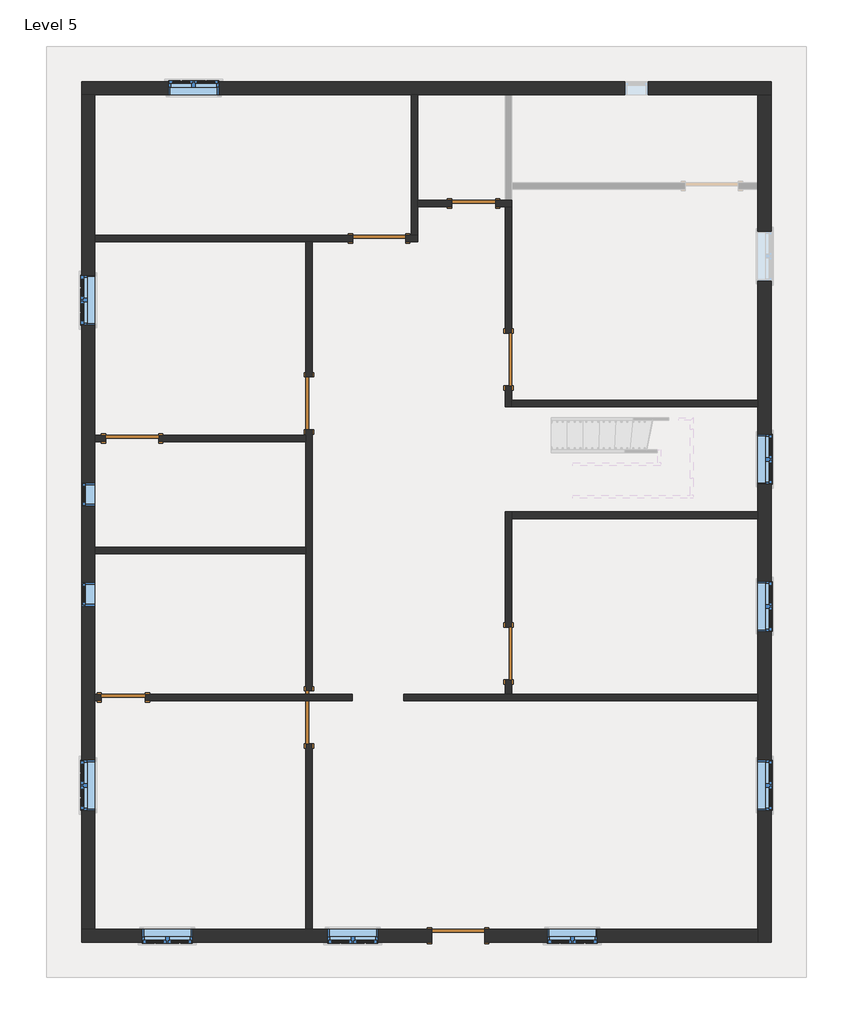
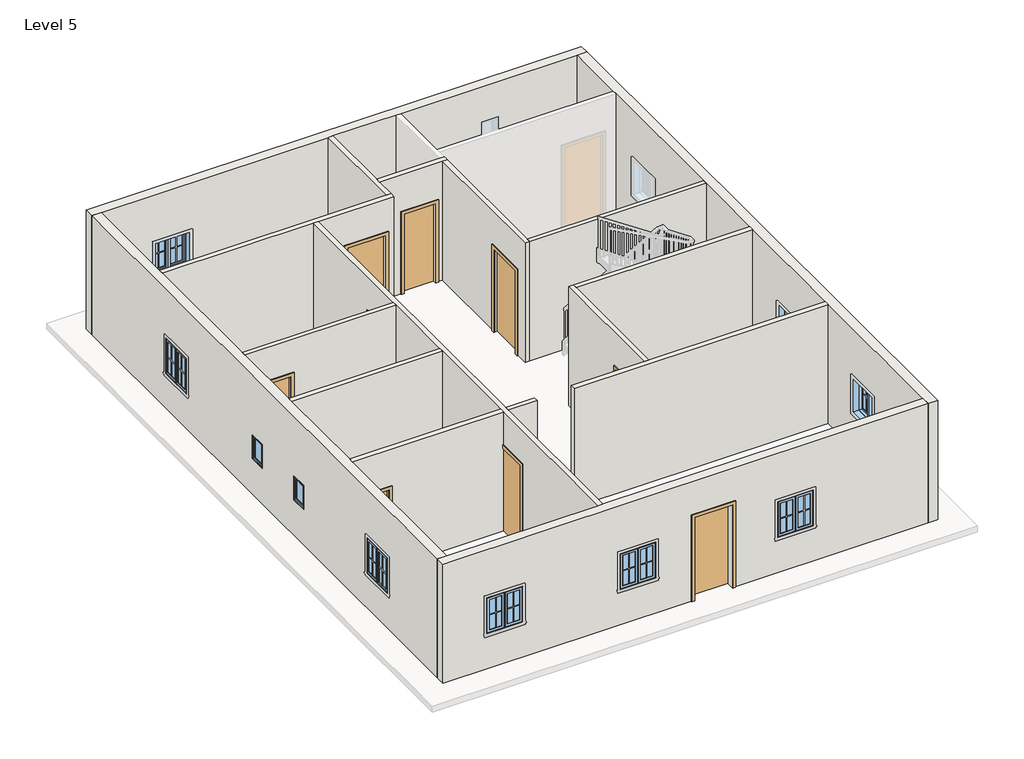
# One storey, part 1 of 3: 16 walls, 11 windows, 9 doors.
"""IFC4 building model written with IfcOpenShell, lengths in millimetres."""

from ifc_helpers import new_model, si_unit, frame, origin, place, context, project, spatial, polyline, outline, extrude, faceted_brep, transform, mapped, element, save
from components import door_d8f5dbb5, door_f2b275c1, door_e5f9f3c4, door_305aa2a5, door_a90ba1ad, window_aa618e30, window_339605e1

model = new_model("IFC4")

# Units and contexts
model_context = context("Model", 3, world=origin())
ifc_project = project(units=[si_unit("LENGTHUNIT", "METRE", prefix="MILLI")], contexts=[model_context])

# Site, building, storey
site = spatial("IfcSite", under=ifc_project)
building = spatial("IfcBuilding", under=site)
storey = spatial("IfcBuildingStorey", under=building, Name="Level 5", Elevation=9601.2)

# Doors
placement = place(None, origin())
door_shape = door_d8f5dbb5(model_context)
element("IfcDoor", 1, ObjectType="Single-Flush : 30\" x 80\"", at=placement, inside=storey, context=model_context, shape_type="MappedRepresentation", body=[
    mapped(door_shape, transform((-509.1743007, 6967.427558, 9601.2), x_axis=(1.0, 0.0, 0.0), y_axis=(0.0, 1.0, 0.0), z_axis=(0.0, 0.0, 1.0))),
])
door_2_shape = door_f2b275c1(model_context)
element("IfcDoor", 2, ObjectType="Single-Flush : 30\" x 80\"", at=placement, inside=storey, context=model_context, shape_type="MappedRepresentation", body=[
    mapped(door_2_shape, transform((-6586.1243007, -1605.072442, 9601.2), x_axis=(-1.0, 0.0, 0.0), y_axis=(0.0, -1.0, 0.0), z_axis=(0.0, 0.0, 1.0))),
])
door_3_shape = door_e5f9f3c4(model_context)
element("IfcDoor", 3, ObjectType="Single-Flush : 36\" x 84\"", at=placement, inside=storey, context=model_context, shape_type="MappedRepresentation", body=[
    mapped(door_3_shape, transform((-2147.4743007, 6357.827558, 9601.2), x_axis=(1.0, 0.0, 0.0), y_axis=(0.0, 1.0, 0.0), z_axis=(0.0, 0.0, 1.0))),
])
element("IfcDoor", 4, ObjectType="Single-Flush : 36\" x 84\"", at=placement, inside=storey, context=model_context, shape_type="MappedRepresentation", body=[
    mapped(door_3_shape, transform((100.4256993, 4262.327558, 9601.2), x_axis=(0.0, -1.0, 0.0), y_axis=(1.0, 0.0, 0.0), z_axis=(0.0, 0.0, 1.0))),
])
element("IfcDoor", 5, ObjectType="Single-Flush : 36\" x 84\"", at=placement, inside=storey, context=model_context, shape_type="MappedRepresentation", body=[
    mapped(door_3_shape, transform((100.4256993, -843.072442, 9601.2), x_axis=(0.0, -1.0, 0.0), y_axis=(1.0, 0.0, 0.0), z_axis=(0.0, 0.0, 1.0))),
])
element("IfcDoor", 6, ObjectType="Single-Flush : 36\" x 84\"", at=placement, inside=storey, context=model_context, shape_type="MappedRepresentation", body=[
    mapped(door_3_shape, transform((-3366.6743007, -1947.972442, 9601.2), x_axis=(0.0, 1.0, 0.0), y_axis=(-1.0, 0.0, 0.0), z_axis=(0.0, 0.0, 1.0))),
])
door_4_shape = door_305aa2a5(model_context)
element("IfcDoor", 7, ObjectType="Single-Flush : 36\" x 84\"", at=placement, inside=storey, context=model_context, shape_type="MappedRepresentation", body=[
    mapped(door_4_shape, transform((-6433.7243007, 2890.727558, 9601.2), x_axis=(-1.0, 0.0, 0.0), y_axis=(0.0, -1.0, 0.0), z_axis=(0.0, 0.0, 1.0))),
])
element("IfcDoor", 8, ObjectType="Single-Flush : 36\" x 84\"", at=placement, inside=storey, context=model_context, shape_type="MappedRepresentation", body=[
    mapped(door_4_shape, transform((-3366.6743007, 3500.327558, 9601.2), x_axis=(0.0, -1.0, 0.0), y_axis=(1.0, 0.0, 0.0), z_axis=(0.0, 0.0, 1.0))),
])
door_5_shape = door_a90ba1ad(model_context)
element("IfcDoor", 9, ObjectType="Single-Flush : 36\" x 84\"", at=placement, inside=storey, context=model_context, shape_type="MappedRepresentation", body=[
    mapped(door_5_shape, transform((-775.8743007, -5738.922442, 9601.2), x_axis=(-1.0, 0.0, 0.0), y_axis=(0.0, -1.0, 0.0), z_axis=(0.0, 0.0, 1.0))),
])

# Walls
element("IfcWall", 10, ObjectType="WALL4.5\"", at=placement, inside=storey, context=model_context, shape_type="Brep", body=[
    faceted_brep([(-1690.2743007, 6300.677558, 11734.8), (-1690.2743007, 6300.677558, 9601.2), (-1480.7243007, 6300.677558, 9601.2), (-1480.7243007, 6300.677558, 12649.2), (-3309.5243007, 6300.677558, 12649.2), (-3423.8243007, 6300.677558, 12649.2), (-7081.4243007, 6300.677558, 12649.2), (-7081.4243007, 6300.677558, 9601.2), (-3423.8243007, 6300.677558, 9601.2), (-3309.5243007, 6300.677558, 9601.2), (-2604.6743007, 6300.677558, 9601.2), (-2604.6743007, 6300.677558, 11734.8), (-1480.7243007, 6414.977558, 9601.2), (-1595.0243007, 6414.977558, 9601.2), (-1690.2743007, 6414.977558, 9601.2), (-1690.2743007, 6414.977558, 11734.8), (-2604.6743007, 6414.977558, 11734.8), (-2604.6743007, 6414.977558, 9601.2), (-7081.4243007, 6414.977558, 9601.2), (-7081.4243007, 6414.977558, 12649.2), (-1595.0243007, 6414.977558, 12649.2), (-1480.7243007, 6414.977558, 12649.2)], [[[0, 1, 2, 3, 4, 5, 6, 7, 8, 9, 10, 11]], [[12, 13, 14, 15, 16, 17, 18, 19, 20, 21]], [[2, 1, 14, 13, 12]], [[10, 9, 8, 7, 18, 17]], [[7, 6, 19, 18]], [[3, 2, 12, 21]], [[15, 14, 1, 0]], [[16, 15, 0, 11]], [[17, 16, 11, 10]], [[6, 5, 4, 3, 21, 20, 19]]]),
])
element("IfcWall", 11, ObjectType="WALL4.5\"", at=placement, inside=storey, context=model_context, shape_type="Brep", body=[
    faceted_brep([(-1480.7243007, 6414.977558, 9601.2), (-1480.7243007, 6910.277558, 9601.2), (-1480.7243007, 7024.577558, 9601.2), (-1480.7243007, 8853.377558, 9601.2), (-1480.7243007, 8853.377558, 12649.2), (-1480.7243007, 7024.577558, 12649.2), (-1480.7243007, 6910.277558, 12649.2), (-1480.7243007, 6414.977558, 12649.2), (-1595.0243007, 6414.977558, 9601.2), (-1595.0243007, 6414.977558, 12649.2), (-1595.0243007, 8853.377558, 12649.2), (-1595.0243007, 8853.377558, 9601.2)], [[[0, 1, 2, 3, 4, 5, 6, 7]], [[8, 9, 10, 11]], [[3, 2, 1, 0, 8, 11]], [[0, 7, 9, 8]], [[4, 3, 11, 10]], [[7, 6, 5, 4, 10, 9]]]),
])
element("IfcWall", 12, ObjectType="WALL4.5\"", at=placement, inside=storey, context=model_context, shape_type="Brep", body=[
    faceted_brep([(-128.1743007, 6910.277558, 11633.2), (-128.1743007, 6910.277558, 9601.2), (43.2756993, 6910.277558, 9601.2), (157.5756993, 6910.277558, 9601.2), (157.5756993, 6910.277558, 12649.2), (43.2756993, 6910.277558, 12649.2), (-1480.7243007, 6910.277558, 12649.2), (-1480.7243007, 6910.277558, 9601.2), (-890.1743007, 6910.277558, 9601.2), (-890.1743007, 6910.277558, 11633.2), (157.5756993, 7024.577558, 9601.2), (43.2756993, 7024.577558, 9601.2), (-128.1743007, 7024.577558, 9601.2), (-128.1743007, 7024.577558, 11633.2), (-890.1743007, 7024.577558, 11633.2), (-890.1743007, 7024.577558, 9601.2), (-1480.7243007, 7024.577558, 9601.2), (-1480.7243007, 7024.577558, 12649.2), (43.2756993, 7024.577558, 12649.2), (157.5756993, 7024.577558, 12649.2)], [[[0, 1, 2, 3, 4, 5, 6, 7, 8, 9]], [[10, 11, 12, 13, 14, 15, 16, 17, 18, 19]], [[8, 7, 16, 15]], [[3, 2, 1, 12, 11, 10]], [[7, 6, 17, 16]], [[4, 3, 10, 19]], [[13, 12, 1, 0]], [[14, 13, 0, 9]], [[15, 14, 9, 8]], [[6, 5, 4, 19, 18, 17]]]),
])
element("IfcWall", 13, ObjectType="WALL4.5\"", at=placement, inside=storey, context=model_context, shape_type="Brep", body=[
    faceted_brep([(-3423.8243007, 3043.127558, 9601.2), (-3423.8243007, 2947.877558, 9601.2), (-3423.8243007, 2833.577558, 9601.2), (-3423.8243007, 1004.777558, 9601.2), (-3423.8243007, 890.477558, 9601.2), (-3423.8243007, -1490.772442, 9601.2), (-3423.8243007, -1490.772442, 11734.8), (-3423.8243007, -1547.922442, 11734.8), (-3423.8243007, -1662.222442, 11734.8), (-3423.8243007, -2405.172442, 11734.8), (-3423.8243007, -2405.172442, 9601.2), (-3423.8243007, -5624.622442, 9601.2), (-3423.8243007, -5624.622442, 12649.2), (-3423.8243007, -1662.222442, 12649.2), (-3423.8243007, -1547.922442, 12649.2), (-3423.8243007, 890.477558, 12649.2), (-3423.8243007, 1004.777558, 12649.2), (-3423.8243007, 2833.577558, 12649.2), (-3423.8243007, 2947.877558, 12649.2), (-3423.8243007, 6300.677558, 12649.2), (-3423.8243007, 6300.677558, 9601.2), (-3423.8243007, 3957.527558, 9601.2), (-3423.8243007, 3957.527558, 11734.8), (-3423.8243007, 3043.127558, 11734.8), (-3309.5243007, -1490.772442, 11734.8), (-3309.5243007, -1490.772442, 9601.2), (-3309.5243007, 3043.127558, 9601.2), (-3309.5243007, 3043.127558, 11734.8), (-3309.5243007, 3957.527558, 11734.8), (-3309.5243007, 3957.527558, 9601.2), (-3309.5243007, 6300.677558, 9601.2), (-3309.5243007, 6300.677558, 12649.2), (-3309.5243007, -1547.922442, 12649.2), (-3309.5243007, -1662.222442, 12649.2), (-3309.5243007, -5624.622442, 12649.2), (-3309.5243007, -5624.622442, 9601.2), (-3309.5243007, -2405.172442, 9601.2), (-3309.5243007, -2405.172442, 11734.8), (-3309.5243007, -1662.222442, 11734.8), (-3309.5243007, -1547.922442, 11734.8)], [[[0, 1, 2, 3, 4, 5, 6, 7, 8, 9, 10, 11, 12, 13, 14, 15, 16, 17, 18, 19, 20, 21, 22, 23]], [[24, 25, 26, 27, 28, 29, 30, 31, 32, 33, 34, 35, 36, 37, 38, 39]], [[21, 20, 30, 29]], [[36, 35, 11, 10]], [[26, 25, 5, 4, 3, 2, 1, 0]], [[12, 11, 35, 34]], [[20, 19, 31, 30]], [[27, 26, 0, 23]], [[28, 27, 23, 22]], [[29, 28, 22, 21]], [[6, 5, 25, 24]], [[9, 8, 7, 6, 24, 39, 38, 37]], [[10, 9, 37, 36]], [[19, 18, 17, 16, 15, 14, 13, 12, 34, 33, 32, 31]]]),
])
element("IfcWall", 14, ObjectType="WALL4.5\"", at=placement, inside=storey, context=model_context, shape_type="Brep", body=[
    faceted_brep([(157.5756993, -1547.922442, 9601.2), (157.5756993, -1300.272442, 9601.2), (157.5756993, -1300.272442, 11734.8), (157.5756993, -385.872442, 11734.8), (157.5756993, -385.872442, 9601.2), (157.5756993, 1500.077558, 9601.2), (157.5756993, 1614.377558, 9601.2), (157.5756993, 1614.377558, 12649.2), (157.5756993, 1500.077558, 12649.2), (157.5756993, -1547.922442, 12649.2), (43.2756993, -1300.272442, 11734.8), (43.2756993, -1300.272442, 9601.2), (43.2756993, -1547.922442, 9601.2), (43.2756993, -1547.922442, 12649.2), (43.2756993, 1614.377558, 12649.2), (43.2756993, 1614.377558, 9601.2), (43.2756993, -385.872442, 9601.2), (43.2756993, -385.872442, 11734.8)], [[[0, 1, 2, 3, 4, 5, 6, 7, 8, 9]], [[10, 11, 12, 13, 14, 15, 16, 17]], [[16, 15, 6, 5, 4]], [[12, 11, 1, 0]], [[7, 6, 15, 14]], [[0, 9, 13, 12]], [[2, 1, 11, 10]], [[3, 2, 10, 17]], [[4, 3, 17, 16]], [[9, 8, 7, 14, 13]]]),
])
element("IfcWall", 15, ObjectType="WALL4.5\"", at=placement, inside=storey, context=model_context, shape_type="SweptSolid", body=[
    extrude(outline(polyline([(4424.7756993, 1500.077558), (157.5756993, 1500.077558), (157.5756993, 1614.377558), (4424.7756993, 1614.377558), (4424.7756993, 1500.077558)])), frame((0.0, 0.0, 9601.2), z_axis=(0.0, 0.0, 1.0), x_axis=(1.0, 0.0, 0.0)), (0.0, 0.0, 1.0), 3048.0),
])
element("IfcWall", 16, ObjectType="WALL4.5\"", at=placement, inside=storey, context=model_context, shape_type="SweptSolid", body=[
    extrude(outline(polyline([(-3423.8243007, 890.477558), (-7081.4243007, 890.477558), (-7081.4243007, 1004.777558), (-3423.8243007, 1004.777558), (-3423.8243007, 890.477558)])), frame((0.0, 0.0, 9601.2), z_axis=(0.0, 0.0, 1.0), x_axis=(1.0, 0.0, 0.0)), (0.0, 0.0, 1.0), 3048.0),
])
element("IfcWall", 17, ObjectType="WALL4.5\"", at=placement, inside=storey, context=model_context, shape_type="SweptSolid", body=[
    extrude(outline(polyline([(9601.2, -7081.4243007), (9601.2, -6890.9243007), (11734.8, -6890.9243007), (11734.8, -5976.5243007), (9601.2, -5976.5243007), (9601.2, -3423.8243007), (12649.2, -3423.8243007), (12649.2, -7081.4243007), (9601.2, -7081.4243007)])), frame((0.0, 2833.577558, 0.0), z_axis=(0.0, 1.0, 0.0), x_axis=(0.0, 0.0, 1.0)), (0.0, 0.0, 1.0), 114.3),
])
element("IfcWall", 18, ObjectType="WALL4.5\"", at=placement, inside=storey, context=model_context, shape_type="Brep", body=[
    faceted_brep([(43.2756993, 3805.127558, 11734.8), (43.2756993, 3805.127558, 9601.2), (43.2756993, 3443.177558, 9601.2), (43.2756993, 3443.177558, 12649.2), (43.2756993, 6910.277558, 12649.2), (43.2756993, 6910.277558, 9601.2), (43.2756993, 4719.527558, 9601.2), (43.2756993, 4719.527558, 11734.8), (157.5756993, 3443.177558, 9601.2), (157.5756993, 3557.477558, 9601.2), (157.5756993, 3805.127558, 9601.2), (157.5756993, 3805.127558, 11734.8), (157.5756993, 4719.527558, 11734.8), (157.5756993, 4719.527558, 9601.2), (157.5756993, 6910.277558, 9601.2), (157.5756993, 6910.277558, 12649.2), (157.5756993, 3557.477558, 12649.2), (157.5756993, 3443.177558, 12649.2)], [[[0, 1, 2, 3, 4, 5, 6, 7]], [[8, 9, 10, 11, 12, 13, 14, 15, 16, 17]], [[6, 5, 14, 13]], [[2, 1, 10, 9, 8]], [[5, 4, 15, 14]], [[3, 2, 8, 17]], [[11, 10, 1, 0]], [[12, 11, 0, 7]], [[13, 12, 7, 6]], [[4, 3, 17, 16, 15]]]),
])
element("IfcWall", 19, ObjectType="WALL4.5\"", at=placement, inside=storey, context=model_context, shape_type="SweptSolid", body=[
    extrude(outline(polyline([(4424.7756993, 3443.177558), (157.5756993, 3443.177558), (157.5756993, 3557.477558), (4424.7756993, 3557.477558), (4424.7756993, 3443.177558)])), frame((0.0, 0.0, 9601.2), z_axis=(0.0, 0.0, 1.0), x_axis=(1.0, 0.0, 0.0)), (0.0, 0.0, 1.0), 3048.0),
])
element("IfcWall", 20, ObjectType="WALL4.5\"", at=placement, inside=storey, context=model_context, shape_type="SweptSolid", body=[
    extrude(outline(polyline([(9601.2, -2614.8628774), (12649.2, -2614.8628774), (12649.2, -3309.5243007), (11734.8, -3309.5243007), (11734.8, -3423.8243007), (12649.2, -3423.8243007), (12649.2, -7081.4243007), (9601.2, -7081.4243007), (9601.2, -6967.1243007), (11633.2, -6967.1243007), (11633.2, -6205.1243007), (9601.2, -6205.1243007), (9601.2, -2614.8628774)])), frame((0.0, -1662.222442, 0.0), z_axis=(0.0, 1.0, 0.0), x_axis=(0.0, 0.0, 1.0)), (0.0, 0.0, 1.0), 114.3),
])
element("IfcWall", 21, ObjectType="WALL4.5\"", at=placement, inside=storey, context=model_context, shape_type="Brep", body=[
    faceted_brep([(-1720.6441625, -1662.222442, 9601.2), (4424.7756993, -1662.222442, 9601.2), (4424.7756993, -1662.222442, 12649.2), (-1720.6441625, -1662.222442, 12649.2), (-1720.6441625, -1547.922442, 9601.2), (-1720.6441625, -1547.922442, 12649.2), (43.2756993, -1547.922442, 12649.2), (157.5756993, -1547.922442, 12649.2), (4424.7756993, -1547.922442, 12649.2), (4424.7756993, -1547.922442, 9601.2), (157.5756993, -1547.922442, 9601.2), (43.2756993, -1547.922442, 9601.2)], [[[0, 1, 2, 3]], [[4, 5, 6, 7, 8, 9, 10, 11]], [[1, 0, 4, 11, 10, 9]], [[0, 3, 5, 4]], [[2, 1, 9, 8]], [[3, 2, 8, 7, 6, 5]]]),
])
element("IfcWall", 22, ObjectType="WALL9\"", at=placement, inside=storey, context=model_context, shape_type="Brep", body=[
    faceted_brep([(-7310.0243007, 8853.377558, 9601.2), (-7081.4243007, 8853.377558, 9601.2), (-1595.0243007, 8853.377558, 9601.2), (-1480.7243007, 8853.377558, 9601.2), (43.2756993, 8853.377558, 9601.2), (157.5756993, 8853.377558, 9601.2), (4424.7756993, 8853.377558, 9601.2), (4653.3756993, 8853.377558, 9601.2), (4653.3756993, 8853.377558, 12649.2), (4424.7756993, 8853.377558, 12649.2), (157.5756993, 8853.377558, 12649.2), (43.2756993, 8853.377558, 12649.2), (-1480.7243007, 8853.377558, 12649.2), (-1595.0243007, 8853.377558, 12649.2), (-7081.4243007, 8853.377558, 12649.2), (-7310.0243007, 8853.377558, 12649.2), (-4935.1243007, 8853.377558, 11430.0), (-4935.1243007, 8853.377558, 10515.6), (-5798.7243007, 8853.377558, 10515.6), (-5798.7243007, 8853.377558, 11430.0), (2522.9506993, 8853.377558, 11734.8), (2522.9506993, 8853.377558, 9906.0), (2116.5506993, 8853.377558, 9906.0), (2116.5506993, 8853.377558, 11734.8), (-7310.0243007, 9081.977558, 9601.2), (-7310.0243007, 9081.977558, 12649.2), (4653.3756993, 9081.977558, 12649.2), (4653.3756993, 9081.977558, 9601.2), (-4935.1243007, 9081.977558, 11430.0), (-5798.7243007, 9081.977558, 11430.0), (-5798.7243007, 9081.977558, 10515.6), (-4935.1243007, 9081.977558, 10515.6), (2522.9506993, 9081.977558, 11734.8), (2116.5506993, 9081.977558, 11734.8), (2116.5506993, 9081.977558, 9906.0), (2522.9506993, 9081.977558, 9906.0)], [[[0, 1, 2, 3, 4, 5, 6, 7, 8, 9, 10, 11, 12, 13, 14, 15], [16, 17, 18, 19], [20, 21, 22, 23]], [[24, 25, 26, 27], [28, 29, 30, 31], [32, 33, 34, 35]], [[7, 6, 5, 4, 3, 2, 1, 0, 24, 27]], [[8, 7, 27, 26]], [[0, 15, 25, 24]], [[17, 16, 28, 31]], [[18, 17, 31, 30]], [[19, 18, 30, 29]], [[16, 19, 29, 28]], [[21, 20, 32, 35]], [[22, 21, 35, 34]], [[23, 22, 34, 33]], [[20, 23, 33, 32]], [[15, 14, 13, 12, 11, 10, 9, 8, 26, 25]]]),
])
element("IfcWall", 23, ObjectType="WALL9\"", at=placement, inside=storey, context=model_context, shape_type="Brep", body=[
    faceted_brep([(4424.7756993, 8853.377558, 9601.2), (4424.7756993, 7329.377558, 9601.2), (4424.7756993, 7215.077558, 9601.2), (4424.7756993, 3557.477558, 9601.2), (4424.7756993, 3443.177558, 9601.2), (4424.7756993, 1614.377558, 9601.2), (4424.7756993, 1500.077558, 9601.2), (4424.7756993, -1547.922442, 9601.2), (4424.7756993, -1662.222442, 9601.2), (4424.7756993, -5624.622442, 9601.2), (4424.7756993, -5853.222442, 9601.2), (4424.7756993, -5853.222442, 12649.2), (4424.7756993, -5624.622442, 12649.2), (4424.7756993, -1662.222442, 12649.2), (4424.7756993, -1547.922442, 12649.2), (4424.7756993, 1500.077558, 12649.2), (4424.7756993, 1614.377558, 12649.2), (4424.7756993, 3443.177558, 12649.2), (4424.7756993, 3557.477558, 12649.2), (4424.7756993, 7215.077558, 12649.2), (4424.7756993, 7329.377558, 12649.2), (4424.7756993, 8853.377558, 12649.2), (4424.7756993, 5621.227558, 11430.0), (4424.7756993, 5621.227558, 10515.6), (4424.7756993, 6484.827558, 10515.6), (4424.7756993, 6484.827558, 11430.0), (4424.7756993, 2096.977558, 11430.0), (4424.7756993, 2096.977558, 10515.6), (4424.7756993, 2960.577558, 10515.6), (4424.7756993, 2960.577558, 11430.0), (4424.7756993, -455.722442, 11430.0), (4424.7756993, -455.722442, 10515.6), (4424.7756993, 407.877558, 10515.6), (4424.7756993, 407.877558, 11430.0), (4424.7756993, -3560.872442, 11430.0), (4424.7756993, -3560.872442, 10515.6), (4424.7756993, -2697.272442, 10515.6), (4424.7756993, -2697.272442, 11430.0), (4653.3756993, 8853.377558, 9601.2), (4653.3756993, 8853.377558, 12649.2), (4653.3756993, -5853.222442, 12649.2), (4653.3756993, -5853.222442, 9601.2), (4653.3756993, 5621.227558, 11430.0), (4653.3756993, 6484.827558, 11430.0), (4653.3756993, 6484.827558, 10515.6), (4653.3756993, 5621.227558, 10515.6), (4653.3756993, 2096.977558, 11430.0), (4653.3756993, 2960.577558, 11430.0), (4653.3756993, 2960.577558, 10515.6), (4653.3756993, 2096.977558, 10515.6), (4653.3756993, -455.722442, 11430.0), (4653.3756993, 407.877558, 11430.0), (4653.3756993, 407.877558, 10515.6), (4653.3756993, -455.722442, 10515.6), (4653.3756993, -3560.872442, 11430.0), (4653.3756993, -2697.272442, 11430.0), (4653.3756993, -2697.272442, 10515.6), (4653.3756993, -3560.872442, 10515.6)], [[[0, 1, 2, 3, 4, 5, 6, 7, 8, 9, 10, 11, 12, 13, 14, 15, 16, 17, 18, 19, 20, 21], [22, 23, 24, 25], [26, 27, 28, 29], [30, 31, 32, 33], [34, 35, 36, 37]], [[38, 39, 40, 41], [42, 43, 44, 45], [46, 47, 48, 49], [50, 51, 52, 53], [54, 55, 56, 57]], [[10, 9, 8, 7, 6, 5, 4, 3, 2, 1, 0, 38, 41]], [[0, 21, 39, 38]], [[11, 10, 41, 40]], [[23, 22, 42, 45]], [[24, 23, 45, 44]], [[25, 24, 44, 43]], [[22, 25, 43, 42]], [[27, 26, 46, 49]], [[28, 27, 49, 48]], [[29, 28, 48, 47]], [[26, 29, 47, 46]], [[31, 30, 50, 53]], [[32, 31, 53, 52]], [[33, 32, 52, 51]], [[30, 33, 51, 50]], [[35, 34, 54, 57]], [[36, 35, 57, 56]], [[37, 36, 56, 55]], [[34, 37, 55, 54]], [[21, 20, 19, 18, 17, 16, 15, 14, 13, 12, 11, 40, 39]]]),
])
element("IfcWall", 24, ObjectType="WALL9\"", at=placement, inside=storey, context=model_context, shape_type="Brep", body=[
    faceted_brep([(-1233.0743007, -5624.622442, 11734.8), (-1233.0743007, -5624.622442, 9601.2), (-3309.5243007, -5624.622442, 9601.2), (-3423.8243007, -5624.622442, 9601.2), (-7081.4243007, -5624.622442, 9601.2), (-7310.0243007, -5624.622442, 9601.2), (-7310.0243007, -5624.622442, 12649.2), (-7081.4243007, -5624.622442, 12649.2), (-3423.8243007, -5624.622442, 12649.2), (-3309.5243007, -5624.622442, 12649.2), (4424.7756993, -5624.622442, 12649.2), (4424.7756993, -5624.622442, 9601.2), (-318.6743007, -5624.622442, 9601.2), (-318.6743007, -5624.622442, 11734.8), (773.5256993, -5624.622442, 11430.0), (773.5256993, -5624.622442, 10515.6), (1637.1256993, -5624.622442, 10515.6), (1637.1256993, -5624.622442, 11430.0), (-3036.4743007, -5624.622442, 11430.0), (-3036.4743007, -5624.622442, 10515.6), (-2172.8743007, -5624.622442, 10515.6), (-2172.8743007, -5624.622442, 11430.0), (-6255.9243007, -5624.622442, 11430.0), (-6255.9243007, -5624.622442, 10515.6), (-5392.3243007, -5624.622442, 10515.6), (-5392.3243007, -5624.622442, 11430.0), (-7310.0243007, -5853.222442, 9601.2), (-1233.0743007, -5853.222442, 9601.2), (-1233.0743007, -5853.222442, 11734.8), (-318.6743007, -5853.222442, 11734.8), (-318.6743007, -5853.222442, 9601.2), (4424.7756993, -5853.222442, 9601.2), (4424.7756993, -5853.222442, 12649.2), (-7310.0243007, -5853.222442, 12649.2), (773.5256993, -5853.222442, 11430.0), (1637.1256993, -5853.222442, 11430.0), (1637.1256993, -5853.222442, 10515.6), (773.5256993, -5853.222442, 10515.6), (-3036.4743007, -5853.222442, 11430.0), (-2172.8743007, -5853.222442, 11430.0), (-2172.8743007, -5853.222442, 10515.6), (-3036.4743007, -5853.222442, 10515.6), (-6255.9243007, -5853.222442, 11430.0), (-5392.3243007, -5853.222442, 11430.0), (-5392.3243007, -5853.222442, 10515.6), (-6255.9243007, -5853.222442, 10515.6)], [[[0, 1, 2, 3, 4, 5, 6, 7, 8, 9, 10, 11, 12, 13], [14, 15, 16, 17], [18, 19, 20, 21], [22, 23, 24, 25]], [[26, 27, 28, 29, 30, 31, 32, 33], [34, 35, 36, 37], [38, 39, 40, 41], [42, 43, 44, 45]], [[12, 11, 31, 30]], [[5, 4, 3, 2, 1, 27, 26]], [[11, 10, 32, 31]], [[6, 5, 26, 33]], [[28, 27, 1, 0]], [[29, 28, 0, 13]], [[30, 29, 13, 12]], [[15, 14, 34, 37]], [[16, 15, 37, 36]], [[17, 16, 36, 35]], [[14, 17, 35, 34]], [[19, 18, 38, 41]], [[20, 19, 41, 40]], [[21, 20, 40, 39]], [[18, 21, 39, 38]], [[23, 22, 42, 45]], [[24, 23, 45, 44]], [[25, 24, 44, 43]], [[22, 25, 43, 42]], [[10, 9, 8, 7, 6, 33, 32]]]),
])
element("IfcWall", 25, ObjectType="WALL9\"", at=placement, inside=storey, context=model_context, shape_type="Brep", body=[
    faceted_brep([(-7081.4243007, -5624.622442, 9601.2), (-7081.4243007, -1662.222442, 9601.2), (-7081.4243007, -1547.922442, 9601.2), (-7081.4243007, 890.477558, 9601.2), (-7081.4243007, 1004.777558, 9601.2), (-7081.4243007, 2833.577558, 9601.2), (-7081.4243007, 2947.877558, 9601.2), (-7081.4243007, 6300.677558, 9601.2), (-7081.4243007, 6414.977558, 9601.2), (-7081.4243007, 8853.377558, 9601.2), (-7081.4243007, 8853.377558, 12649.2), (-7081.4243007, 6414.977558, 12649.2), (-7081.4243007, 6300.677558, 12649.2), (-7081.4243007, 2947.877558, 12649.2), (-7081.4243007, 2833.577558, 12649.2), (-7081.4243007, 1004.777558, 12649.2), (-7081.4243007, 890.477558, 12649.2), (-7081.4243007, -1547.922442, 12649.2), (-7081.4243007, -1662.222442, 12649.2), (-7081.4243007, -5624.622442, 12649.2), (-7081.4243007, 388.827558, 11125.2), (-7081.4243007, 388.827558, 10515.6), (-7081.4243007, -17.572442, 10515.6), (-7081.4243007, -17.572442, 11125.2), (-7081.4243007, 2122.377558, 11125.2), (-7081.4243007, 2122.377558, 10515.6), (-7081.4243007, 1715.977558, 10515.6), (-7081.4243007, 1715.977558, 11125.2), (-7081.4243007, 5722.827558, 11430.0), (-7081.4243007, 5722.827558, 10515.6), (-7081.4243007, 4859.227558, 10515.6), (-7081.4243007, 4859.227558, 11430.0), (-7081.4243007, -2697.272442, 11430.0), (-7081.4243007, -2697.272442, 10515.6), (-7081.4243007, -3560.872442, 10515.6), (-7081.4243007, -3560.872442, 11430.0), (-7310.0243007, -5624.622442, 9601.2), (-7310.0243007, -5624.622442, 12649.2), (-7310.0243007, 8853.377558, 12649.2), (-7310.0243007, 8853.377558, 9601.2), (-7310.0243007, 388.827558, 11125.2), (-7310.0243007, -17.572442, 11125.2), (-7310.0243007, -17.572442, 10515.6), (-7310.0243007, 388.827558, 10515.6), (-7310.0243007, 2122.377558, 11125.2), (-7310.0243007, 1715.977558, 11125.2), (-7310.0243007, 1715.977558, 10515.6), (-7310.0243007, 2122.377558, 10515.6), (-7310.0243007, 5722.827558, 11430.0), (-7310.0243007, 4859.227558, 11430.0), (-7310.0243007, 4859.227558, 10515.6), (-7310.0243007, 5722.827558, 10515.6), (-7310.0243007, -2697.272442, 11430.0), (-7310.0243007, -3560.872442, 11430.0), (-7310.0243007, -3560.872442, 10515.6), (-7310.0243007, -2697.272442, 10515.6)], [[[0, 1, 2, 3, 4, 5, 6, 7, 8, 9, 10, 11, 12, 13, 14, 15, 16, 17, 18, 19], [20, 21, 22, 23], [24, 25, 26, 27], [28, 29, 30, 31], [32, 33, 34, 35]], [[36, 37, 38, 39], [40, 41, 42, 43], [44, 45, 46, 47], [48, 49, 50, 51], [52, 53, 54, 55]], [[9, 8, 7, 6, 5, 4, 3, 2, 1, 0, 36, 39]], [[10, 9, 39, 38]], [[0, 19, 37, 36]], [[21, 20, 40, 43]], [[22, 21, 43, 42]], [[23, 22, 42, 41]], [[20, 23, 41, 40]], [[25, 24, 44, 47]], [[26, 25, 47, 46]], [[27, 26, 46, 45]], [[24, 27, 45, 44]], [[29, 28, 48, 51]], [[30, 29, 51, 50]], [[31, 30, 50, 49]], [[28, 31, 49, 48]], [[33, 32, 52, 55]], [[34, 33, 55, 54]], [[35, 34, 54, 53]], [[32, 35, 53, 52]], [[19, 18, 17, 16, 15, 14, 13, 12, 11, 10, 38, 37]]]),
])

# Windows
window_shape = window_aa618e30(model_context)
element("IfcWindow", 26, ObjectType="Fixed : 16\" x 24\"", at=placement, inside=storey, context=model_context, shape_type="MappedRepresentation", body=[
    mapped(window_shape, transform((-7195.7243007, 223.727558, 9601.2), x_axis=(0.0, 1.0, 0.0), y_axis=(-1.0, 0.0, 0.0), z_axis=(0.0, 0.0, 1.0))),
])
element("IfcWindow", 27, ObjectType="Fixed : 16\" x 24\"", at=placement, inside=storey, context=model_context, shape_type="MappedRepresentation", body=[
    mapped(window_shape, transform((-7195.7243007, 1957.277558, 9601.2), x_axis=(0.0, 1.0, 0.0), y_axis=(-1.0, 0.0, 0.0), z_axis=(0.0, 0.0, 1.0))),
])
window_2_shape = window_339605e1(model_context)
element("IfcWindow", 28, ObjectType="Window-Casement-Double : 34\" x 36\"", at=placement, inside=storey, context=model_context, shape_type="MappedRepresentation", body=[
    mapped(window_2_shape, transform((-5366.9243007, 8967.677558, 9601.2), x_axis=(1.0, 0.0, 0.0), y_axis=(0.0, 1.0, 0.0), z_axis=(0.0, 0.0, 1.0))),
])
element("IfcWindow", 29, ObjectType="Window-Casement-Double : 34\" x 36\"", at=placement, inside=storey, context=model_context, shape_type="MappedRepresentation", body=[
    mapped(window_2_shape, transform((-7195.7243007, 5291.027558, 9601.2), x_axis=(0.0, 1.0, 0.0), y_axis=(-1.0, 0.0, 0.0), z_axis=(0.0, 0.0, 1.0))),
])
element("IfcWindow", 30, ObjectType="Window-Casement-Double : 34\" x 36\"", at=placement, inside=storey, context=model_context, shape_type="MappedRepresentation", body=[
    mapped(window_2_shape, transform((4539.0756993, 2528.777558, 9601.2), x_axis=(0.0, -1.0, 0.0), y_axis=(1.0, 0.0, 0.0), z_axis=(0.0, 0.0, 1.0))),
])
element("IfcWindow", 31, ObjectType="Window-Casement-Double : 34\" x 36\"", at=placement, inside=storey, context=model_context, shape_type="MappedRepresentation", body=[
    mapped(window_2_shape, transform((4539.0756993, -23.922442, 9601.2), x_axis=(0.0, -1.0, 0.0), y_axis=(1.0, 0.0, 0.0), z_axis=(0.0, 0.0, 1.0))),
])
element("IfcWindow", 32, ObjectType="Window-Casement-Double : 34\" x 36\"", at=placement, inside=storey, context=model_context, shape_type="MappedRepresentation", body=[
    mapped(window_2_shape, transform((4539.0756993, -3129.072442, 9601.2), x_axis=(0.0, -1.0, 0.0), y_axis=(1.0, 0.0, 0.0), z_axis=(0.0, 0.0, 1.0))),
])
element("IfcWindow", 33, ObjectType="Window-Casement-Double : 34\" x 36\"", at=placement, inside=storey, context=model_context, shape_type="MappedRepresentation", body=[
    mapped(window_2_shape, transform((1205.3256993, -5738.922442, 9601.2), x_axis=(-1.0, 0.0, 0.0), y_axis=(0.0, -1.0, 0.0), z_axis=(0.0, 0.0, 1.0))),
])
element("IfcWindow", 34, ObjectType="Window-Casement-Double : 34\" x 36\"", at=placement, inside=storey, context=model_context, shape_type="MappedRepresentation", body=[
    mapped(window_2_shape, transform((-2604.6743007, -5738.922442, 9601.2), x_axis=(-1.0, 0.0, 0.0), y_axis=(0.0, -1.0, 0.0), z_axis=(0.0, 0.0, 1.0))),
])
element("IfcWindow", 35, ObjectType="Window-Casement-Double : 34\" x 36\"", at=placement, inside=storey, context=model_context, shape_type="MappedRepresentation", body=[
    mapped(window_2_shape, transform((-5824.1243007, -5738.922442, 9601.2), x_axis=(-1.0, 0.0, 0.0), y_axis=(0.0, -1.0, 0.0), z_axis=(0.0, 0.0, 1.0))),
])
element("IfcWindow", 36, ObjectType="Window-Casement-Double : 34\" x 36\"", at=placement, inside=storey, context=model_context, shape_type="MappedRepresentation", body=[
    mapped(window_2_shape, transform((-7195.7243007, -3129.072442, 9601.2), x_axis=(0.0, 1.0, 0.0), y_axis=(-1.0, 0.0, 0.0), z_axis=(0.0, 0.0, 1.0))),
])

save(model, "model.ifc")

# Revit data of these elements
# Type "Single-Flush : 30\" x 80\""
#   Type Mark = "5"
#   Construction Type Id = "MDOOR"
#   Assembly Code = "C1020"
#   Analytic Construction = "Metal"
#   Thickness = 0' - 2"
#   Heat Transfer Coefficient (U) = 0.651978 BTU/(h·ft²·°F)
#   Height = 6' - 8"
#   Trim Projection Ext = 0' - 1"
#   Trim Projection Int = 0' - 1"
#   Trim Width = 0' - 3"
#   Width = 2' - 6"
#   Define Thermal Properties by = 1
#   Define Thermal Properties by = 1
#   Door Material = Door - Panel
#   Frame Material = Door - Frame
#   Visual Light Transmittance = 0
#   Solar Heat Gain Coefficient = 0
#   Function = (empty or 0)
#   Wall Closure = (empty or 0)
# Type "Single-Flush : 36\" x 84\""
#   Type Mark = "1"
#   Construction Type Id = "MDOOR"
#   Assembly Code = "C1020"
#   Analytic Construction = "Metal"
#   Thickness = 0' - 2"
#   Heat Transfer Coefficient (U) = 0.651978 BTU/(h·ft²·°F)
#   Height = 7' - 0"
#   Trim Projection Ext = 0' - 1"
#   Trim Projection Int = 0' - 1"
#   Trim Width = 0' - 3"
#   Width = 3' - 0"
#   Define Thermal Properties by = 1
#   Define Thermal Properties by = 1
#   Door Material = Door - Panel
#   Frame Material = Door - Frame
#   Visual Light Transmittance = 0
#   Solar Heat Gain Coefficient = 0
#   Function = (empty or 0)
#   Wall Closure = (empty or 0)
# Type "WALL4.5\""
#   Assembly Code = "B2010"
#   Layers, outside or top first: 0' - 4 1/2" no material (function 1)
# Type "WALL9\""
#   Assembly Code = "B2010"
#   Layers, outside or top first: 0' - 9" no material (function 1)
# Type "Fixed : 16\" x 24\""
#   Type Mark = "4"
#   Construction Type Id = "GSP4R"
#   Assembly Code = "B2020100"
#   Analytic Construction = "1/8 in Pilkington single glazing"
#   Visual Light Transmittance = 0.9
#   Solar Heat Gain Coefficient = 0.78
#   Heat Transfer Coefficient (U) = 0.6496 BTU/(h·ft²·°F)
#   Height = 2' - 0"
#   Default Sill Height = 3' - 0"
#   Width = 1' - 4"
#   Window Inset = 0' - 0 3/4"
#   Define Thermal Properties by = 1
#   Define Thermal Properties by = 1
#   Glass Pane Material = Glass
#   Sash Material = Sash
#   Wall Closure = (empty or 0)
# Type "Window-Casement-Double : 34\" x 36\""
#   Type Mark = "14"
#   Fire Rating = "0.5h"
#   Assembly Code = "B2020100"
#   Analytic Construction = "Double glazing - domestic"
#   Frame Extension [instance default] = 0' - 0 1/4"
#   Window Inset [instance default] = 0' - 0"
#   Wall Thickness [instance default] = 0' - 6"
#   Interior Wall Closure [instance default] = 0' - 2 1/4"
#   Half Width = 1' - 5"
#   Visual Light Transmittance = 0.81
#   Thermal Resistance (R) = 1.8146 (h·ft²·°F)/BTU
#   Solar Heat Gain Coefficient = 0.76
#   Rough Width = 2' - 10 1/2"
#   Rough Height = 3' - 0 1/2"
#   Height = 3' - 0"
#   Heat Transfer Coefficient (U) = 0.5511 BTU/(h·ft²·°F)
#   Exterior Wall Closure [instance default] = 0' - 1 1/4"
#   Extension Jamb [instance default] = 0' - 2 1/4"
#   Default Sill Height = 3' - 0"
#   Width = 2' - 10"
#   Define Thermal Properties by = 0
#   Muntin Visibility = yes
#   Interior Trim Visibility [instance default] = yes
#   Exterior Trim Visibility [instance default] = yes
#   Extension Jamb Visibility [instance default] = yes
#   Interior Trim Material = Wood - Stained
#   Muntin Pattern = Muntin Pattern_2x2 : Muntin Pattern_2x2
#   Interior Trim = Trim-Window-Interior-Flat : Picture Frame
#   Interior Frame Material = Wood - Stained
#   Glass Panel Material = Glass
#   Exterior Trim Material = Clad - White
#   Exterior Trim = Trim-Window-Exterior-Flat : with Sill
#   Exterior Frame Material = Clad - White
#   Wall Closure = (empty or 0)
# Elements 1, 2 (IfcDoor, "Single-Flush : 30\" x 80\"")
#   Phase Created = New Construction
#   Materials on its faces: "Door - Frame", "Door - Panel"
# Elements 3, 4, 5, 6, 7, 8, 9 (IfcDoor, "Single-Flush : 36\" x 84\"")
#   Phase Created = New Construction
#   Materials on its faces: "Door - Frame", "Door - Panel"
# Elements 10, 11, 12, 13, 14, 15, 16, 17, 18, 19, 20, 21 (IfcWall, "WALL4.5\"")
#   Top Offset = 0' - 0"
#   Base Offset = 0' - 0"
#   Unconnected Height = 10' - 0"
#   wall height = 10' - 0"
#   Phase Created = New Construction
#   Base Constraint = Level 5
#   Materials on its faces: "Default Wall"
# Elements 22, 23, 24, 25 (IfcWall, "WALL9\"")
#   Top Offset = 0' - 0"
#   Base Offset = 0' - 0"
#   Unconnected Height = 10' - 0"
#   wall height = 10' - 0"
#   Phase Created = New Construction
#   Base Constraint = Level 5
#   Materials on its faces: "Default Wall"
# Element 26 (IfcWindow, "Fixed : 16\" x 24\"")
#   Mark = "41"
#   Phase Created = New Construction
#   Materials on its faces: "Sash", "Glass"
# Element 27 (IfcWindow, "Fixed : 16\" x 24\"")
#   Mark = "43"
#   Phase Created = New Construction
#   Materials on its faces: "Sash", "Glass"
# Element 28 (IfcWindow, "Window-Casement-Double : 34\" x 36\"")
#   Mark = "42"
#   Window Inset = 0' - 0"
#   Interior Wall Closure = 0' - 2 1/4"
#   Frame Extension = 0' - 0 1/4"
#   Exterior Wall Closure = 0' - 1 1/4"
#   Interior Trim Visibility = yes
#   Exterior Trim Visibility = yes
#   Phase Created = New Construction
#   Materials on its faces: "Wood - Stained", "Glass", "Clad - White"
# Element 29 (IfcWindow, "Window-Casement-Double : 34\" x 36\"")
#   Mark = "44"
#   Window Inset = 0' - 0"
#   Interior Wall Closure = 0' - 2 1/4"
#   Frame Extension = 0' - 0 1/4"
#   Exterior Wall Closure = 0' - 1 1/4"
#   Interior Trim Visibility = yes
#   Exterior Trim Visibility = yes
#   Phase Created = New Construction
#   Materials on its faces: "Wood - Stained", "Glass", "Clad - White"
# Element 30 (IfcWindow, "Window-Casement-Double : 34\" x 36\"")
#   Mark = "46"
#   Window Inset = 0' - 0"
#   Interior Wall Closure = 0' - 2 1/4"
#   Frame Extension = 0' - 0 1/4"
#   Exterior Wall Closure = 0' - 1 1/4"
#   Interior Trim Visibility = yes
#   Exterior Trim Visibility = yes
#   Phase Created = New Construction
#   Materials on its faces: "Wood - Stained", "Glass", "Clad - White"
# Element 31 (IfcWindow, "Window-Casement-Double : 34\" x 36\"")
#   Mark = "47"
#   Window Inset = 0' - 0"
#   Interior Wall Closure = 0' - 2 1/4"
#   Frame Extension = 0' - 0 1/4"
#   Exterior Wall Closure = 0' - 1 1/4"
#   Interior Trim Visibility = yes
#   Exterior Trim Visibility = yes
#   Phase Created = New Construction
#   Materials on its faces: "Wood - Stained", "Glass", "Clad - White"
# Element 32 (IfcWindow, "Window-Casement-Double : 34\" x 36\"")
#   Mark = "48"
#   Window Inset = 0' - 0"
#   Interior Wall Closure = 0' - 2 1/4"
#   Frame Extension = 0' - 0 1/4"
#   Exterior Wall Closure = 0' - 1 1/4"
#   Interior Trim Visibility = yes
#   Exterior Trim Visibility = yes
#   Phase Created = New Construction
#   Materials on its faces: "Wood - Stained", "Glass", "Clad - White"
# Element 33 (IfcWindow, "Window-Casement-Double : 34\" x 36\"")
#   Mark = "49"
#   Window Inset = 0' - 0"
#   Interior Wall Closure = 0' - 2 1/4"
#   Frame Extension = 0' - 0 1/4"
#   Exterior Wall Closure = 0' - 1 1/4"
#   Interior Trim Visibility = yes
#   Exterior Trim Visibility = yes
#   Phase Created = New Construction
#   Materials on its faces: "Wood - Stained", "Glass", "Clad - White"
# Element 34 (IfcWindow, "Window-Casement-Double : 34\" x 36\"")
#   Mark = "50"
#   Window Inset = 0' - 0"
#   Interior Wall Closure = 0' - 2 1/4"
#   Frame Extension = 0' - 0 1/4"
#   Exterior Wall Closure = 0' - 1 1/4"
#   Interior Trim Visibility = yes
#   Exterior Trim Visibility = yes
#   Phase Created = New Construction
#   Materials on its faces: "Wood - Stained", "Glass", "Clad - White"
# Element 35 (IfcWindow, "Window-Casement-Double : 34\" x 36\"")
#   Mark = "51"
#   Window Inset = 0' - 0"
#   Interior Wall Closure = 0' - 2 1/4"
#   Frame Extension = 0' - 0 1/4"
#   Exterior Wall Closure = 0' - 1 1/4"
#   Interior Trim Visibility = yes
#   Exterior Trim Visibility = yes
#   Phase Created = New Construction
#   Materials on its faces: "Wood - Stained", "Glass", "Clad - White"
# Element 36 (IfcWindow, "Window-Casement-Double : 34\" x 36\"")
#   Mark = "52"
#   Window Inset = 0' - 0"
#   Interior Wall Closure = 0' - 2 1/4"
#   Frame Extension = 0' - 0 1/4"
#   Exterior Wall Closure = 0' - 1 1/4"
#   Interior Trim Visibility = yes
#   Exterior Trim Visibility = yes
#   Phase Created = New Construction
#   Materials on its faces: "Wood - Stained", "Glass", "Clad - White"
# Materials
#   "Door - Panel": class "Wood", colour RGB 210 159 95, transparency 0, Cost = 0
#   "Door - Frame": colour RGB 118 70 51, transparency 0, Cost = 0
#   "Glass": class "Glass", colour RGB 0 128 192, transparency 0.75, Description = "Soda Lime Glass", Cost = 0
#   "Sash": class "Wood", colour RGB 224 178 126, transparency 0, Cost = 0
#   "Wood - Stained": class "Wood", colour RGB 224 178 126, transparency 0, Cost = 0
#   "Clad - White": class "Wood", colour RGB 242 242 238, transparency 0, Cost = 0
#   "Default Wall": colour RGB 128 128 128, transparency 0, Cost = 0
